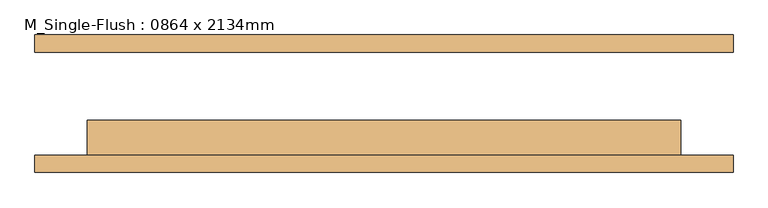
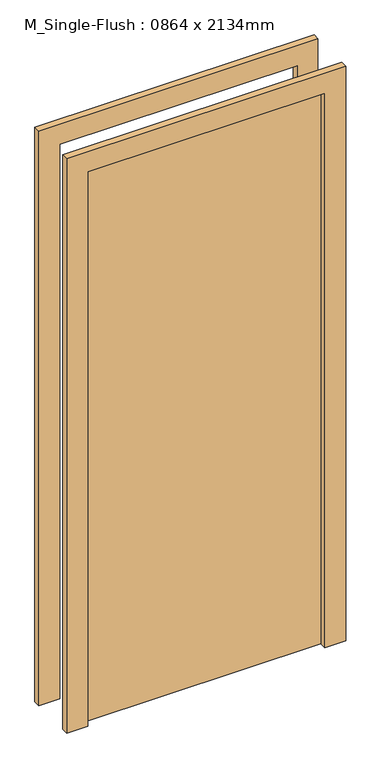
"""IFC4 building model written with IfcOpenShell, lengths in millimetres: door geometry, M_Single-Flush : 0864 x 2134mm."""

from ifc_helpers import new_model, si_unit, frame, origin, origin_with_axes, place, context, project, spatial, polyline, outline, extrude, source, transform, mapped, element, save


def m_single_flush_0864_x_2134mm_0748c0c9(model_context):
    return source(origin(), model_context, "Body", "SweptSolid", [
        extrude(outline(polyline([(2210.0, -508.0), (0.0, -508.0), (0.0, -432.0), (2134.0, -432.0), (2134.0, 432.0), (0.0, 432.0), (0.0, 508.0), (2210.0, 508.0), (2210.0, -508.0)])), frame((0.0, -100.0, 0.0), z_axis=(0.0, 1.0, 0.0), x_axis=(0.0, 0.0, 1.0)), (0.0, 0.0, 1.0), 25.0),
        extrude(outline(polyline([(2210.0, 508.0), (2210.0, -508.0), (0.0, -508.0), (0.0, -432.0), (2134.0, -432.0), (2134.0, 432.0), (0.0, 432.0), (0.0, 508.0), (2210.0, 508.0)])), frame((0.0, 75.0, 0.0), z_axis=(0.0, 1.0, 0.0), x_axis=(0.0, 0.0, 1.0)), (0.0, 0.0, 1.0), 25.0),
        extrude(outline(polyline([(432.0, -24.0), (432.0, -75.0), (-432.0, -75.0), (-432.0, -24.0), (432.0, -24.0)])), origin_with_axes(), (0.0, 0.0, 1.0), 2134.0),
    ])


if __name__ == "__main__":
    model = new_model("IFC4")
    model_context = context("Model", 3, world=origin())
    ifc_project = project(units=[si_unit("LENGTHUNIT", "METRE", prefix="MILLI")], contexts=[model_context])
    site = spatial("IfcSite", under=ifc_project)
    building = spatial("IfcBuilding", under=site)
    placement = place(None, origin())
    m_single_flush_0864_x_2134mm_shape = m_single_flush_0864_x_2134mm_0748c0c9(model_context)
    element("IfcDoor", 1, ObjectType="M_Single-Flush : 0864 x 2134mm", at=placement, inside=building, context=model_context, shape_type="MappedRepresentation", body=[
        mapped(m_single_flush_0864_x_2134mm_shape, transform((0.0, 0.0, 0.0), x_axis=(1.0, 0.0, 0.0), y_axis=(0.0, 1.0, 0.0), z_axis=(0.0, 0.0, 1.0))),
    ])
    save(model, "model.ifc")

# Revit data of these elements
# Type "M_Single-Flush : 0864 x 2134mm"
#   Type Mark = "16"
#   Thickness = 51 mm
#   Height = 2134 mm
#   Trim Projection Ext = 25 mm
#   Trim Projection Int = 25 mm
#   Trim Width = 76 mm
#   Width = 864 mm
#   Door Material = Door - Panel
#   Frame Material = Door - Frame
#   Function = (empty or 0)
#   Wall Closure = (empty or 0)
# Element 1 (IfcDoor, "M_Single-Flush : 0864 x 2134mm")
#   Materials on its faces: "Door - Frame", "Door - Panel"
# Materials
#   "Door - Panel": class "Wood", colour RGB 114 82 51, transparency 0
#   "Door - Frame": colour RGB 153 76 43, transparency 0
